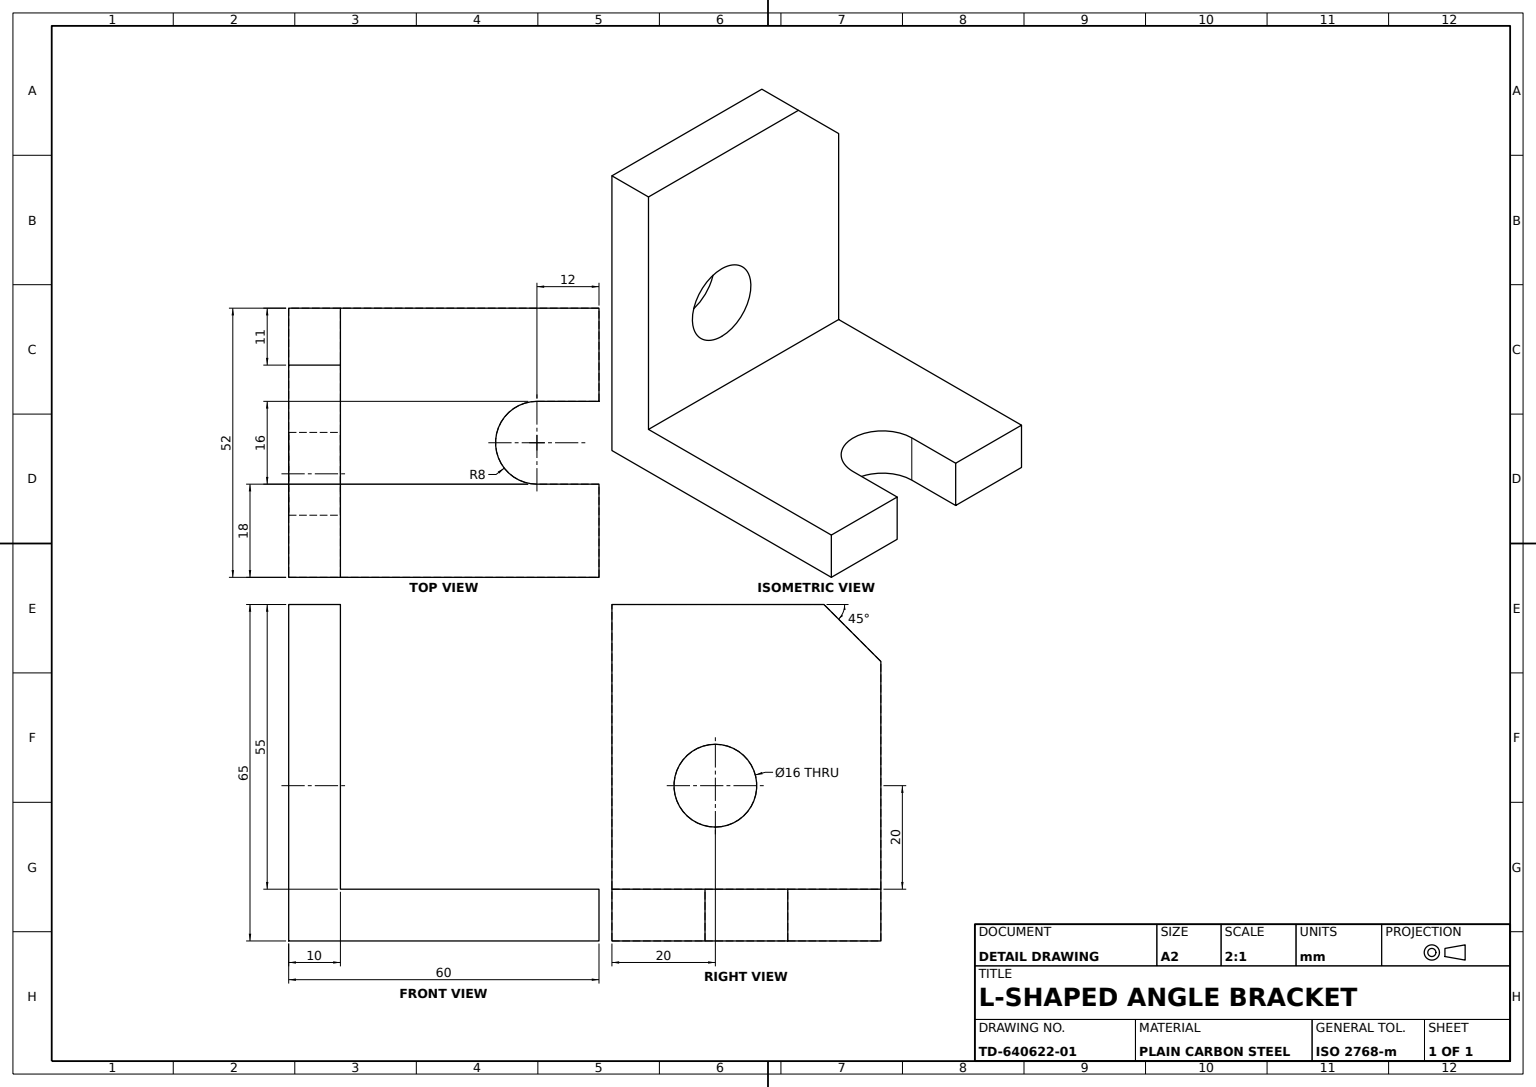
from build123d import *

# Parameters (mm, degrees)
L_BRACKET_BODY_DEPTH  = 26
BASE_U_SLOT_DEPTH     = 86.44588931
UPRIGHT_HOLE_SKETCH_R = 8
UPRIGHT_HOLE_16_DEPTH = 87.029064856
CHAMFER_11X45_SIZE    = 11


with BuildPart() as part:
    # L-Profile Sketch → L-Bracket Body (new, symmetric)
    with BuildSketch(Plane.XY):
        Polygon((0, 0), (0, 65), (10, 65), (10, 10), (60, 10), (60, 0), align=None)
    extrude(amount=L_BRACKET_BODY_DEPTH, both=True)

    # Base Slot Sketch → Base U-Slot (cut, through all)
    with BuildSketch(Plane(origin=(0, 10, 0), x_dir=(1, 0, 0), z_dir=(0, 1, 0))):
        with BuildLine():
            Line((48, 8), (60, 8))
            Line((60, 8), (60, -8))
            Line((60, -8), (48, -8))
            ThreePointArc((48, -8), (40, 0), (48, 8))
        make_face()
    extrude(amount=-BASE_U_SLOT_DEPTH, mode=Mode.SUBTRACT)

    # Upright Hole Sketch → Upright Hole Ø16 (cut, through all)
    with BuildSketch(Plane(origin=(10, 0, 0), x_dir=(0, 0, -1), z_dir=(1, 0, 0))):
        with Locations(Location((-6, 30, 0), (0, 0, 90))):
            Circle(UPRIGHT_HOLE_SKETCH_R)
    extrude(amount=-UPRIGHT_HOLE_16_DEPTH, mode=Mode.SUBTRACT)

    # Chamfer 11x45°
    chamfer_11x45_edges = [part.edges().sort_by_distance(p)[0] for p in [
        (5, 65, -26),
    ]]
    chamfer(chamfer_11x45_edges, length=CHAMFER_11X45_SIZE)


solid = part.part
